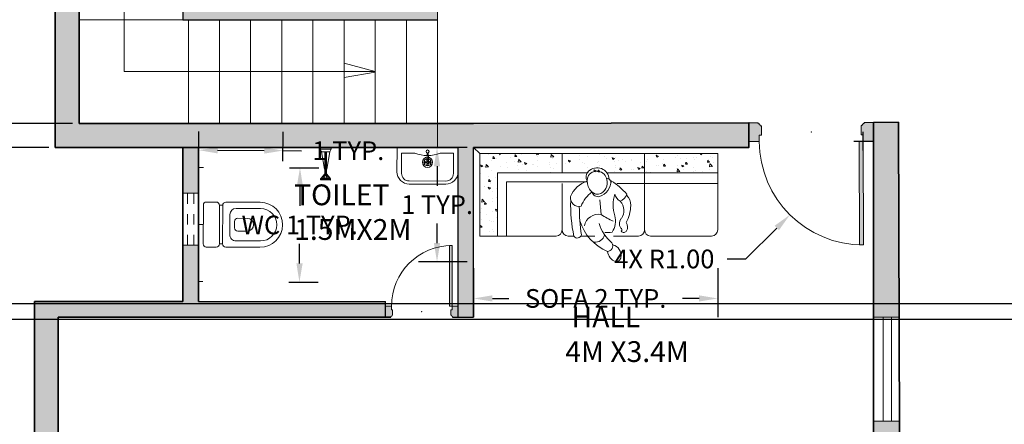
# Model space of a CAD drawing. Units: metres. Extents: x 2031 to 2061.8, y 1886.4 to 1909.8.
# Tile 3 of 10: x 2036.4 to 2045.9, y 1892.7 to 1896.6. Entities that reach past the tile are written whole.
import ezdxf

# ---------------------------------------------------------------- set-up
doc = ezdxf.new("R2010")
doc.units = ezdxf.units.M
doc.linetypes.add('DASHED', pattern=[0.75, 0.5, -0.25])
for name, color, linetype, lineweight in [('A-ANNO-DIMS', 2, 'Continuous', 18), ('A-AREA-IDEN', 7, 'Continuous', 18), ('A-FLOR-FIXT', 8, 'Continuous', 18), ('A-FLOR-STRS', 7, 'Continuous', 18), ('A-FLOR-STRS-PATH', 1, 'Continuous', 13), ('A-GLAZ-OVHD', 30, 'DASHED', 13), ('A-WALL-PATT', 252, 'Continuous', 13), ('doors & windows', 30, 'Continuous', 18), ('furniture', 24, 'Continuous', 13), ('inner walls', 4, 'Continuous', 25), ('windows', 30, 'Continuous', 18)]:
    doc.layers.add(name, color=color, linetype=linetype, lineweight=lineweight)
doc.layers.add('outer walls', color=1, linetype='Continuous', lineweight=35, plot=False)
doc.styles.get("Standard").update_dxf_attribs({"font": 'arial.ttf'})
doc.dimstyles.get("Standard").update_dxf_attribs({"dimtxt": 0.18, "dimasz": 0.18, "dimexe": 0.18, "dimexo": 0.0625, "dimgap": 0.09, "dimtad": 0, "dimtih": 1, "dimtoh": 1, "dimdec": 4, "dimzin": 0, "dimdsep": 46, "dimtxsty": 'Standard', "dimcen": 0.09, "dimadec": 0, "dimazin": 0, "dimtfac": 1, "dimtdec": 4, "dimtofl": 0, "dimtmove": 0, "dimatfit": 3, "dimfxl": 1, "dimtolj": 1, "dimtzin": 0, "dimarcsym": 0})

# ---------------------------------------------------------------- blocks, each defined once
blk = doc.blocks.new('D2')
at = {"layer": 'doors & windows'}
h = blk.add_hatch(dxfattribs=at)
h.set_pattern_fill('DOTS', color=256, scale=2, angle=180, style=0)
h.set_pattern_definition([(180, (0, -4), (-0.0625, -0.125), [0, -0.125])])
h.paths.add_polyline_path([(2.5, 0), (3.5, 0), (3.5, 24.98, 0.010003), (2.5, 25)])
h = blk.add_hatch(dxfattribs=at)
h.set_pattern_fill('DOTS', color=256, scale=2, angle=180, style=0)
h.set_pattern_definition([(180, (0, 0), (-0.0625, -0.125), [0, -0.125])])
edge = h.paths.add_edge_path()
edge.add_line((27.5, 0), (27.5, -1.5))
edge.add_line((27.5, -1.5), (27, -1.5))
edge.add_line((27, -1.5), (27, -3.75))
edge.add_line((27, -3.75), (27.25, -3.75))
edge.add_arc((27.76, -3.74), 0.509, 181.0059, 268.9941)
edge.add_line((27.75, -4.25), (27.75, -4.5))
edge.add_line((27.75, -4.5), (30, -4.5))
edge.add_line((30, -4.5), (30, 0))
edge.add_line((30, 0), (27.5, 0))
edge = h.paths.add_edge_path()
edge.add_line((2.5, -1.5), (2.5, 0))
edge.add_line((2.5, 0), (0, 0))
edge.add_line((0, 0), (0, -4.5))
edge.add_line((0, -4.5), (2.25, -4.5))
edge.add_line((2.25, -4.5), (2.25, -4.25))
edge.add_arc((2.24, -3.74), 0.509, 271.0059, 358.9941)
edge.add_line((2.75, -3.75), (3, -3.75))
edge.add_line((3, -3.75), (3, -1.5))
edge.add_line((3, -1.5), (2.5, -1.5))
for p, q in [((0, 0), (0, -4.5)), ((30, 0), (30, -4.5))]:
    blk.add_line(p, q)
blk.add_lwpolyline([(3.5, 0), (3.5, 25), (2.5, 25), (2.5, 0)], close=True, dxfattribs=at)
for points in [[(3, -3.75), (3, -1.5), (2.5, -1.5), (2.5, 0), (0, 0)], [(27, -3.75), (27, -1.5), (27.5, -1.5), (27.5, 0), (30, 0)], [(0, -4.5), (2.25, -4.5)], [(30, -4.5), (27.75, -4.5)]]:
    blk.add_lwpolyline(points, dxfattribs=at)
for points in [[(2.25, -4.5), (2.25, -4.25, 0.403966), (2.75, -3.75), (3, -3.75)], [(27.75, -4.5), (27.75, -4.25, -0.403966), (27.25, -3.75), (27, -3.75)]]:
    blk.add_lwpolyline(points, format="xyb", dxfattribs=at)
at = {"layer": 'doors & windows', "ltscale": 6}
blk.add_arc((2.5, 0), 25, 0, 90, dxfattribs=at)
at = {"layer": 'doors & windows'}
blk.add_point((15, -2.25), dxfattribs=at)
blk = doc.blocks.new('MAN')
at = {"layer": 'doors & windows'}
blk.add_line((1.3, -9.85), (0.89, -5.45), dxfattribs=at)
for centre, radius, start, end in [((-0.81, 1.3), 2.37, 132.7993, 210.1219), ((0, 0), 3.06, 359.7942, 144.0351), ((0.1, 0.48), 3.6, 2.8928, 134.5528), ((-0.36, -7.56), 8.07, 108.0153, 157.5724), ((1.3, 0.05), 4.16, 155.2349, 248.5051), ((-0.98, 0.55), 5.34, 289.2819, 356.6237), ((2.86, -0.44), 1.38, 352.7443, 87.7525), ((-8.99, -19.77), 24.04, 41.647, 56.3067), ((-0.1, -0.61), 3.22, 267.7788, 10.6507), ((-5.32, -4.92), 2.54, 170.002, 284.7527), ((34.75, -7.19), 42.53, 177.9613, 192.4551), ((4.14, -10.82), 9.46, 125.6851, 158.6987), ((0.38, -2.75), 1.79, 192.3382, 283.0231), ((15.87, -7.04), 10.97, 162.7002, 196.7262), ((8.59, -3.01), 3.29, 193.5598, 239.9446), ((5.83, -2.73), 3.32, 289.6374, 341.2911), ((3.84, -8.67), 4.24, 325.4363, 41.8446), ((6.12, -7.03), 4.01, 358.2671, 46.939), ((54.76, -7.35), 59.95, 180.1044, 188.2297), ((-0.78, -6.94), 10.91, 330.7562, 358.8997), ((9.03, -7.36), 14.72, 197.1765, 246.7641), ((0.5, -14.05), 4.27, 79.2575, 168.509), ((16.49, 13.41), 27.78, 236.8487, 245.427), ((-0.19, -11.81), 5.78, 325.2412, 16.1794), ((8.85, -12.54), 2.12, 136.0875, 215.1077), ((12.84, -8.62), 12.77, 197.9012, 229.3504), ((6.8, -14.37), 0.689, 315.9836, 61.7947), ((7.06, -13.61), 2.15, 328.4119, 38.6474), ((-5.78, -15.61), 1.25, 217.214, 345.0614), ((-0.4, -15.27), 2.81, 261.6005, 345.5998), ((3.21, -8.72), 6.53, 262.8142, 281.931), ((8.05, -14.12), 1.05, 224.0636, 323.687), ((3.09, -19.2), 1.68, 274.444, 31.8659), ((4.09, -22.01), 3.16, 349.15, 77.9716), ((6.99, -20.36), 3.8, 187.9766, 248.0432), ((5.75, -22.44), 1.45, 262.6631, 353.5986)]:
    blk.add_arc(centre, radius, start, end, dxfattribs=at)
blk = doc.blocks.new('sofa 2')
at = {"layer": 'furniture', "ltscale": 0.5}
h = blk.add_hatch(dxfattribs=at)
h.set_pattern_fill('AR-CONC', color=256, angle=450, style=0)
h.set_pattern_definition([(40, (-1099.1507, 871.655), (-0.627521, 7.172602), [0.75, -8.25]), (95, (-1099.151, 871.655), (7.52192, -1.387513), [0.6, -6.6]), (349.5486, (-1099.203, 872.253), (6.894395, 5.785094), [0.637402, -7.01142]), (43.8158, (-1097.151, 871.655), (-1.65519, 10.67241), [1.125, -12.375]), (353.3644, (-1097.289, 872.544), (9.74118, 9.34663), [0.9561, -10.51713]), (98.8158, (-1097.151, 871.655), (9.74119, 9.34662), [0.9, -9.9]), (69, (-1097.6507, 872.655), (-4.02619, 5.96907), [0.75, -8.25]), (124, (-1097.651, 872.655), (7.2515, 2.433153), [0.6, -6.6]), (18.5486, (-1097.986, 873.1524), (3.225305, 8.402226), [0.637402, -7.01142]), (52.5, (-1099.1507, 871.655), (3.3289385, 0.1215986), [0, -6.52, 0, -6.7, 0, -6.625]), (82.5, (-1099.1507, 871.655), (3.944117, 2.630695), [0, -3.82, 0, -6.37, 0, -2.525]), (122.5, (-1099.1507, 869.425), (-0.2255487, 5.3382244), [0, -2.5, 0, -7.8, 0, -10.35]), (132.5, (-1099.1507, 868.425), (1.00105, 5.831862), [0, -3.25, 0, -5.18, 0, -7.35])])
h.paths.add_polyline_path([(-8.27, -37.7, 0.168872), (-7.9, -36.76, 0.613808), (-6.95, -30.77, 0.074869), (-8.27, -30.38), (-8.27, -29), (-2, -29), (-2, -56), (-8.27, -56)])
h.paths.add_polyline_path([(-8.27, -7.77), (-29, -7.77), (-29, -2), (-2, -2), (-2, -29), (-8.27, -29)])
h.paths.add_polyline_path([(-8.27, -80), (-2, -80), (-2, -56), (-8.27, -56)])
at = {"layer": 'furniture'}
for p, q in [((-2, -2), (0, 0)), ((-29, -2), (-2, -2)), ((-29, -27), (-29, -2)), ((-2, -2), (-2, -80)), ((-8.27, -7.77), (-29, -7.77)), ((-8.27, -37.27), (-8.27, -7.77)), ((-11.27, -10.77), (-29, -10.77)), ((-11.27, -37.27), (-11.27, -10.77)), ((-27, -29), (-11.8, -29)), ((-8.27, -29), (-2, -29)), ((-29, -32.87), (-29, -31)), ((-29, -39.74), (-29, -35.16)), ((-8.27, -37.7), (-8.27, -37.7)), ((-8.27, -43.66), (-8.27, -80)), ((-29, -45.8), (-29, -54)), ((-11.8, -80), (-11.8, -46.89)), ((-29, -78), (-29, -58)), ((-27, -56), (-2, -56)), ((-2, -80), (-27, -80))]:
    blk.add_line(p, q, dxfattribs=at)
for centre, start, end in [((-27, -27), 180, 270), ((-27, -31), 90, 180), ((-27, -54), 180, 270), ((-27, -58), 90, 180), ((-27, -78), 180, 270)]:
    blk.add_arc(centre, 2, start, end, dxfattribs=at)
at = {"xscale": 1.099999999999999, "yscale": 1.099999999999999, "zscale": 1.099999999999999, "rotation": 270}
blk.add_blockref('MAN', (-11.13, -40.34), dxfattribs=at)
blk = doc.blocks.new('commode')
for p, q in [((-7.09, 19.41), (-7.09, 8.61)), ((-5.09, 11.81), (-5.09, 19.57)), ((5.09, 11.81), (5.09, 19.57)), ((7.09, 19.41), (7.09, 8.61)), ((-2, 12.37), (-2, 15.37)), ((2, 12.37), (2, 15.37)), ((-3.15, 9.87), (3.15, 9.87)), ((-1, 11.37), (1, 11.37)), ((-6.09, 7.61), (6.09, 7.61)), ((-6.09, 6.61), (-6.09, 7.61)), ((-6.09, 6.61), (6.09, 6.61)), ((6.09, 7.61), (6.09, 6.61)), ((-7.09, 2.5), (-7.09, 5.61)), ((7.09, 2.5), (7.09, 5.61)), ((-18, 1.5), (-18, 0)), ((-6.09, 1.5), (6.09, 1.5)), ((0, 1.5), (0, 0)), ((18, 1.5), (18, 0))]:
    blk.add_line(p, q)
for centre, radius, start, end in [((0, 19.41), 7.09, 0, 180), ((0, 19.57), 5.09, 0, 180), ((0, 15.37), 2, 0, 180), ((-3.15, 11.81), 1.94, 180, 270), ((-1, 12.37), 1, 180, 270), ((1, 12.37), 1, 270, 0), ((3.15, 11.81), 1.94, 270, 0), ((-6.09, 8.61), 1, 180, 270), ((-6.09, 5.61), 1, 90, 180), ((6.09, 8.61), 1, 270, 0), ((6.09, 5.61), 1, 0, 90), ((-6.09, 2.5), 1, 180, 270), ((6.09, 2.5), 1, 270, 0)]:
    blk.add_arc(centre, radius, start, end)
blk = doc.blocks.new('wash basin 1')
for p, q in [((0, 10), (-8, 10)), ((0, 10), (0, -10)), ((-8.5, 8.5), (-1.85, 8.5)), ((-1.85, 8.5), (-1.85, 4.19)), ((-12, 6), (-12, -6)), ((-11, 6), (-11, -6)), ((-1.85, -8.5), (-1.85, -4.19)), ((-8.5, -8.5), (-1.85, -8.5)), ((0, -10), (-8, -10))]:
    blk.add_line(p, q)
blk.add_lwpolyline([(-1.83, 0.11), (-5.25, 0.25), (-5.23, -0.38), (-1.8, -0.19)])
for centre, radius in [((-4.87, 0), 1.68), ((-4.87, 0), 1.18), ((-5.63, 0), 0.25), ((-4.87, 0.75), 0.25), ((-4.87, 0), 0.25), ((-4.19, 0), 0.25), ((-1.34, 0), 0.5), ((-4.87, -0.72), 0.25)]:
    blk.add_circle(centre, radius)
for centre, radius, start, end in [((-8, 6), 4, 90, 180), ((-8.5, 6), 2.5, 90, 180), ((8.89, 0), 11.53, 158.7059, 201.2941), ((-8, -6), 4, 180, 270), ((-8.5, -6), 2.5, 180, 270)]:
    blk.add_arc(centre, radius, start, end)
blk = doc.blocks.new('tap & shower')
for p, q in [((1.71, 0), (-1.71, 0)), ((-1.71, 0), (-1.71, -0.5)), ((1.71, 0), (1.71, -0.5)), ((1.71, -0.5), (-1.71, -0.5)), ((1.31, -1.4), (-1.31, -1.4)), ((-1.31, -1.4), (-0.39, -7)), ((-0.32, -0.5), (0.32, -0.5)), ((-0.27, -7.94), (-0.27, -1.4)), ((-0.22, -7.94), (-0.22, -1.4)), ((-0.16, -7.94), (-0.16, -1.4)), ((0, -8.48), (0, -1.4)), ((0.16, -7.94), (0.16, -1.4)), ((0.22, -7.94), (0.22, -1.4)), ((0.27, -7.94), (0.27, -1.4)), ((0.39, -7), (1.31, -1.4)), ((-1.48, -9.96), (-0.27, -8.48)), ((-0.21, -8.48), (-0.94, -9.96)), ((-0.09, -8.48), (-0.4, -9.96)), ((-0.32, -7.94), (0.32, -7.94)), ((-0.32, -8.48), (-0.32, -7.94)), ((-0.32, -8.48), (0.32, -8.48)), ((0.09, -8.48), (0.4, -9.96)), ((0.21, -8.48), (0.94, -9.96)), ((1.48, -9.96), (0.27, -8.48)), ((0.32, -8.48), (0.32, -7.94)), ((-1.62, -10.37), (-1.62, -10.1)), ((-1.48, -9.96), (1.48, -9.96)), ((-1.48, -10.5), (-1.48, -9.96)), ((-1.48, -10.5), (1.48, -10.5)), ((-1.43, -10.5), (-1.43, -9.96)), ((-1.37, -10.5), (-1.37, -9.96)), ((-1.32, -10.5), (-1.32, -9.96)), ((-1.27, -10.5), (-1.27, -9.96)), ((-1.21, -10.5), (-1.21, -9.96)), ((-1.16, -10.5), (-1.16, -9.96)), ((-1.1, -10.5), (-1.1, -9.96)), ((-1.05, -10.5), (-1.05, -9.96)), ((-1, -10.5), (-1, -9.96)), ((-0.94, -10.5), (-0.94, -9.96)), ((-0.89, -10.5), (-0.89, -9.96)), ((-0.84, -10.5), (-0.84, -9.96)), ((-0.78, -10.5), (-0.78, -9.96)), ((-0.73, -10.5), (-0.73, -9.96)), ((-0.67, -10.5), (-0.67, -9.96)), ((-0.62, -10.5), (-0.62, -9.96)), ((-0.57, -10.5), (-0.57, -9.96)), ((-0.51, -10.5), (-0.51, -9.96)), ((-0.46, -10.5), (-0.46, -9.96)), ((-0.4, -10.5), (-0.4, -9.96)), ((-0.35, -10.5), (-0.35, -9.96)), ((-0.3, -10.5), (-0.3, -9.96)), ((-0.24, -10.5), (-0.24, -9.96)), ((-0.19, -10.5), (-0.19, -9.96)), ((-0.13, -10.5), (-0.13, -9.96)), ((-0.08, -10.5), (-0.08, -9.96)), ((-0.03, -10.5), (-0.03, -9.96)), ((0.03, -10.5), (0.03, -9.96)), ((0.08, -10.5), (0.08, -9.96)), ((0.13, -10.5), (0.13, -9.96)), ((0.19, -10.5), (0.19, -9.96)), ((0.24, -10.5), (0.24, -9.96)), ((0.3, -10.5), (0.3, -9.96)), ((0.35, -10.5), (0.35, -9.96)), ((0.4, -10.5), (0.4, -9.96)), ((0.46, -10.5), (0.46, -9.96)), ((0.51, -10.5), (0.51, -9.96)), ((0.57, -10.5), (0.57, -9.96)), ((0.62, -10.5), (0.62, -9.96)), ((0.67, -10.5), (0.67, -9.96)), ((0.73, -10.5), (0.73, -9.96)), ((0.78, -10.5), (0.78, -9.96)), ((0.84, -10.5), (0.84, -9.96)), ((0.89, -10.5), (0.89, -9.96)), ((0.94, -10.5), (0.94, -9.96)), ((1, -10.5), (1, -9.96)), ((1.05, -10.5), (1.05, -9.96)), ((1.1, -10.5), (1.1, -9.96)), ((1.16, -10.5), (1.16, -9.96)), ((1.21, -10.5), (1.21, -9.96)), ((1.27, -10.5), (1.27, -9.96)), ((1.32, -10.5), (1.32, -9.96)), ((1.37, -10.5), (1.37, -9.96)), ((1.43, -10.5), (1.43, -9.96)), ((1.48, -10.5), (1.48, -9.96)), ((1.62, -10.37), (1.62, -10.1))]:
    blk.add_line(p, q)
for centre, radius, start, end in [((-0.02, -0.29), 1.7, 187.1825, 220.9028), ((0.02, -0.29), 1.7, 319.0972, 352.8175), ((0, -6.99), 0.392, 181.7992, 358.2008), ((-1.48, -10.1), 0.135, 90, 180), ((-1.48, -10.37), 0.135, 180, 270), ((1.48, -10.1), 0.135, 0, 90), ((1.48, -10.37), 0.135, 270, 0)]:
    blk.add_arc(centre, radius, start, end)
blk = doc.blocks.new('*D30')
at = {"layer": 'A-ANNO-DIMS', "color": 0, "lineweight": -2, "transparency": 16777216}
for p, q in [((2038.9882, 1895.1459), (2039.2707, 1895.1445)), ((2039.0898, 1894.9654), (2039.0889, 1894.7784)), ((2039.0862, 1894.2253), (2039.0871, 1894.4123)), ((2038.9828, 1894.0458), (2039.2653, 1894.0444))]:
    blk.add_line(p, q, dxfattribs=at)
at = {"layer": 'A-ANNO-DIMS', "color": 0, "transparency": 16777216}
for points in [[(2039.0598, 1894.9655), (2039.1198, 1894.9652), (2039.0907, 1895.1454)], [(2039.0562, 1894.2254), (2039.1162, 1894.2251), (2039.0853, 1894.0453)]]:
    blk.add_solid(points, dxfattribs=at)
at = {"layer": 'Defpoints', "color": 0, "transparency": 16777216}
for p in [(2038.9257, 1895.1462), (2038.9203, 1894.0461), (2039.0853, 1894.0453)]:
    blk.add_point(p, dxfattribs=at)
at = {"layer": 'A-ANNO-DIMS', "color": 0, "transparency": 16777216, "insert": (2039.088, 1894.5953), "char_height": 0.18, "attachment_point": 5}
blk.add_mtext('\\A1;WC 1 TYP.', dxfattribs=at)
blk = doc.blocks.new('*D31')
at = {"layer": 'A-ANNO-DIMS', "color": 0, "lineweight": -2, "transparency": 16777216}
for p, q in [((2038.1162, 1895.2127), (2038.1176, 1895.4952)), ((2038.926, 1895.2087), (2038.9274, 1895.4912)), ((2038.2967, 1895.3143), (2038.7465, 1895.3121)), ((2038.9265, 1895.3112), (2039.1065, 1895.3103))]:
    blk.add_line(p, q, dxfattribs=at)
at = {"layer": 'A-ANNO-DIMS', "color": 0, "transparency": 16777216}
for points in [[(2038.2969, 1895.3443), (2038.2966, 1895.2843), (2038.1167, 1895.3152)], [(2038.7467, 1895.3421), (2038.7464, 1895.2821), (2038.9265, 1895.3112)]]:
    blk.add_solid(points, dxfattribs=at)
at = {"layer": 'Defpoints', "color": 0, "transparency": 16777216}
for p in [(2038.9265, 1895.3112), (2038.1159, 1895.1502), (2038.9257, 1895.1462)]:
    blk.add_point(p, dxfattribs=at)
at = {"layer": 'A-ANNO-DIMS', "color": 0, "transparency": 16777216, "insert": (2039.5562, 1895.3103), "char_height": 0.18, "attachment_point": 5}
blk.add_mtext('\\A1;1 TYP.', dxfattribs=at)
blk = doc.blocks.new('*D34')
at = {"layer": 'A-ANNO-DIMS', "color": 0, "lineweight": -2, "transparency": 16777216}
for p, q in [((2040.7632, 1894.1783), (2040.7632, 1893.7082)), ((2043.1138, 1894.1783), (2043.1138, 1893.7082)), ((2040.9432, 1893.8882), (2041.1035, 1893.8882)), ((2042.9338, 1893.8882), (2042.7735, 1893.8882))]:
    blk.add_line(p, q, dxfattribs=at)
at = {"layer": 'A-ANNO-DIMS', "color": 0, "transparency": 16777216}
for points in [[(2040.9432, 1893.9182), (2040.9432, 1893.8582), (2040.7632, 1893.8882)], [(2042.9338, 1893.9182), (2042.9338, 1893.8582), (2043.1138, 1893.8882)]]:
    blk.add_solid(points, dxfattribs=at)
at = {"layer": 'Defpoints', "color": 0, "transparency": 16777216}
for p in [(2040.7632, 1894.2408), (2043.1138, 1894.2408), (2040.7632, 1893.8882)]:
    blk.add_point(p, dxfattribs=at)
at = {"layer": 'A-ANNO-DIMS', "color": 0, "transparency": 16777216, "insert": (2041.9385, 1893.8882), "char_height": 0.18, "attachment_point": 5}
blk.add_mtext('\\A1;SOFA 2 TYP.', dxfattribs=at)
blk = doc.blocks.new('*D35')
at = {"layer": 'A-ANNO-DIMS', "color": 0, "lineweight": -2, "transparency": 16777216}
for p, q in [((2040.7007, 1895.3412), (2040.2306, 1895.3412)), ((2040.4106, 1895.1612), (2040.4106, 1894.9714)), ((2040.4106, 1894.4208), (2040.4106, 1894.6106)), ((2040.7007, 1894.2408), (2040.2306, 1894.2408))]:
    blk.add_line(p, q, dxfattribs=at)
at = {"layer": 'A-ANNO-DIMS', "color": 0, "transparency": 16777216}
for points in [[(2040.3806, 1895.1612), (2040.4406, 1895.1612), (2040.4106, 1895.3412)], [(2040.3806, 1894.4208), (2040.4406, 1894.4208), (2040.4106, 1894.2408)]]:
    blk.add_solid(points, dxfattribs=at)
at = {"layer": 'Defpoints', "color": 0, "transparency": 16777216}
for p in [(2040.4106, 1895.3412), (2040.7632, 1895.3412), (2040.7632, 1894.2408)]:
    blk.add_point(p, dxfattribs=at)
at = {"layer": 'A-ANNO-DIMS', "color": 0, "transparency": 16777216, "insert": (2040.4106, 1894.791), "char_height": 0.18, "attachment_point": 5}
blk.add_mtext('\\A1;1 TYP.', dxfattribs=at)
blk = doc.blocks.new('*D44')
at = {"layer": 'A-ANNO-DIMS', "color": 0, "lineweight": -2, "transparency": 16777216}
for p, q in [((2036.2328, 1900.7199), (2036.2328, 1886.3902)), ((2056.4539, 1889.9931), (2056.4539, 1886.3902)), ((2036.4128, 1886.5702), (2045.949, 1886.5702)), ((2056.2739, 1886.5702), (2046.7377, 1886.5702))]:
    blk.add_line(p, q, dxfattribs=at)
at = {"layer": 'A-ANNO-DIMS', "color": 0, "transparency": 16777216}
for points in [[(2036.4128, 1886.6002), (2036.4128, 1886.5402), (2036.2328, 1886.5702)], [(2056.2739, 1886.6002), (2056.2739, 1886.5402), (2056.4539, 1886.5702)]]:
    blk.add_solid(points, dxfattribs=at)
at = {"layer": 'Defpoints', "color": 0, "transparency": 16777216}
for p in [(2036.2328, 1900.7824), (2056.4539, 1890.0556), (2056.4539, 1886.5702)]:
    blk.add_point(p, dxfattribs=at)
at = {"layer": 'A-ANNO-DIMS', "color": 0, "transparency": 16777216, "insert": (2046.3433, 1886.5702), "char_height": 0.18, "attachment_point": 5}
blk.add_mtext('\\A1;20.22', dxfattribs=at)
blk = doc.blocks.new('*D51')
at = {"layer": 'A-ANNO-DIMS', "color": 0, "lineweight": -2, "transparency": 16777216}
for p, q in [((2036.9007, 1899.3712), (2031.5648, 1899.3712)), ((2031.7448, 1899.1912), (2031.7448, 1897.6532)), ((2031.7448, 1895.7512), (2031.7448, 1897.2892)), ((2036.9007, 1895.5712), (2031.5648, 1895.5712))]:
    blk.add_line(p, q, dxfattribs=at)
at = {"layer": 'A-ANNO-DIMS', "color": 0, "transparency": 16777216}
for points in [[(2031.7148, 1899.1912), (2031.7748, 1899.1912), (2031.7448, 1899.3712)], [(2031.7148, 1895.7512), (2031.7748, 1895.7512), (2031.7448, 1895.5712)]]:
    blk.add_solid(points, dxfattribs=at)
at = {"layer": 'Defpoints', "color": 0, "transparency": 16777216}
for p in [(2031.7448, 1899.3712), (2036.9632, 1899.3712), (2036.9632, 1895.5712)]:
    blk.add_point(p, dxfattribs=at)
at = {"layer": 'A-ANNO-DIMS', "color": 0, "transparency": 16777216, "insert": (2031.7448, 1897.4712), "char_height": 0.18, "attachment_point": 5}
blk.add_mtext('\\A1;3.8', dxfattribs=at)
blk = doc.blocks.new('*D54')
at = {"layer": 'A-ANNO-DIMS', "color": 0, "lineweight": -2, "transparency": 16777216}
for p, q in [((2036.6707, 1895.3412), (2031.5648, 1895.3412)), ((2031.7448, 1895.1612), (2031.7448, 1892.892)), ((2031.7448, 1890.2591), (2031.7448, 1892.5282)), ((2036.4707, 1890.0791), (2031.5648, 1890.0791))]:
    blk.add_line(p, q, dxfattribs=at)
at = {"layer": 'A-ANNO-DIMS', "color": 0, "transparency": 16777216}
for points in [[(2031.7148, 1895.1612), (2031.7748, 1895.1612), (2031.7448, 1895.3412)], [(2031.7148, 1890.2591), (2031.7748, 1890.2591), (2031.7448, 1890.0791)]]:
    blk.add_solid(points, dxfattribs=at)
at = {"layer": 'Defpoints', "color": 0, "transparency": 16777216}
for p in [(2036.7332, 1895.3412), (2031.7448, 1890.0791), (2036.5332, 1890.0791)]:
    blk.add_point(p, dxfattribs=at)
at = {"layer": 'A-ANNO-DIMS', "color": 0, "transparency": 16777216, "insert": (2031.7448, 1892.7101), "char_height": 0.18, "attachment_point": 5}
blk.add_mtext('\\A1;5.262', dxfattribs=at)
blk = doc.blocks.new('*D61')
at = {"layer": 'A-ANNO-DIMS', "color": 0, "lineweight": -2, "transparency": 16777216}
for p, q in [((2031.7448, 1894.0148), (2031.7448, 1894.1948)), ((2031.7448, 1894.1948), (2031.9248, 1894.1948)), ((2052.1275, 1893.8348), (2031.5648, 1893.8348)), ((2051.9775, 1893.6848), (2031.5648, 1893.6848)), ((2031.7448, 1893.5048), (2031.7448, 1893.3248))]:
    blk.add_line(p, q, dxfattribs=at)
at = {"layer": 'A-ANNO-DIMS', "color": 0, "transparency": 16777216}
for points in [[(2031.7148, 1894.0148), (2031.7748, 1894.0148), (2031.7448, 1893.8348)], [(2031.7148, 1893.5048), (2031.7748, 1893.5048), (2031.7448, 1893.6848)]]:
    blk.add_solid(points, dxfattribs=at)
at = {"layer": 'Defpoints', "color": 0, "transparency": 16777216}
for p in [(2031.7448, 1893.8348), (2052.19, 1893.8348), (2052.04, 1893.6848)]:
    blk.add_point(p, dxfattribs=at)
at = {"layer": 'A-ANNO-DIMS', "color": 0, "transparency": 16777216, "insert": (2032.2492, 1894.1948), "char_height": 0.18, "attachment_point": 5}
blk.add_mtext('\\A1;0.15', dxfattribs=at)
blk = doc.blocks.new('*D64')
at = {"layer": 'A-ANNO-DIMS', "color": 0, "lineweight": -2, "transparency": 16777216}
for p, q in [((2044.5141, 1895.3129), (2044.5141, 1895.4929)), ((2044.4241, 1895.4029), (2044.6041, 1895.4029)), ((2043.3857, 1894.2683), (2043.6819, 1894.5662)), ((2043.2057, 1894.2683), (2043.3857, 1894.2683))]:
    blk.add_line(p, q, dxfattribs=at)
at = {"layer": 'A-ANNO-DIMS', "color": 0, "transparency": 16777216}
blk.add_solid([(2043.6606, 1894.5873), (2043.7032, 1894.545), (2043.8088, 1894.6938)], dxfattribs=at)
at = {"layer": 'Defpoints', "color": 0, "transparency": 16777216}
for p in [(2044.5141, 1895.4029), (2043.8088, 1894.6938)]:
    blk.add_point(p, dxfattribs=at)
at = {"layer": 'A-ANNO-DIMS', "color": 0, "transparency": 16777216, "insert": (2042.5991, 1894.2683), "char_height": 0.18, "attachment_point": 5}
blk.add_mtext('\\A1;4X R1.00', dxfattribs=at)

msp = doc.modelspace()

# ---------------------------------------------------------------- hatches: boundary and pattern name
at = {"layer": 'A-WALL-PATT'}
h = msp.add_hatch(color=256, dxfattribs=at)
h.dxf.hatch_style = 1
h.paths.add_polyline_path([(2036.9632, 1899.3712), (2037.9632, 1899.3712), (2037.9631, 1899.6012), (2036.7332, 1899.6012), (2036.7332, 1895.3412), (2040.4157, 1895.3412), (2040.4157, 1895.5712), (2038.0157, 1895.5712), (2036.9632, 1895.5712), (2036.9632, 1896.5712), (2036.9632, 1898.3712)])
h.paths.add_polyline_path([(2038.0632, 1898.2712), (2040.4157, 1898.2712), (2040.4157, 1898.3712), (2037.9632, 1898.3712), (2037.9632, 1896.5712), (2040.4157, 1896.5712), (2040.4157, 1896.6712), (2038.0632, 1896.6712)], flags=17)
h = msp.add_hatch(color=256, dxfattribs=at)
h.dxf.hatch_style = 1
h.paths.add_polyline_path([(2036.7632, 1893.709), (2039.9132, 1893.709), (2039.9132, 1893.859), (2038.1132, 1893.859), (2038.1132, 1894.4001), (2037.9632, 1894.4001), (2037.9632, 1893.859), (2036.5332, 1893.859), (2036.5332, 1892.3865), (2036.7632, 1892.3865)])
h.paths.add_polyline_path([(2038.1132, 1895.3412), (2037.9632, 1895.3412), (2037.9632, 1894.9001), (2038.1132, 1894.9001)])
h.paths.add_polyline_path([(2043.4132, 1895.5795), (2040.7632, 1895.5712), (2040.4157, 1895.5712), (2040.4157, 1895.3412), (2040.6132, 1895.3412), (2040.6132, 1893.709), (2040.7632, 1893.709), (2040.7632, 1895.3412), (2043.4139, 1895.3412)])
h.paths.add_polyline_path([(2039.7057, 1890.309), (2036.7632, 1890.309), (2036.7632, 1891.1865), (2036.5332, 1891.1865), (2036.5332, 1890.079), (2038.4982, 1890.079), (2038.4982, 1888.429), (2038.6482, 1888.429), (2038.6482, 1890.079), (2039.7057, 1890.079)])
h.paths.add_polyline_path([(2042.7749, 1889.8182), (2042.6136, 1889.8182), (2042.6136, 1891.8182), (2042.6136, 1891.9682), (2042.4636, 1891.9682), (2041.6986, 1891.9682), (2041.6986, 1891.8182), (2042.4636, 1891.8182), (2042.4636, 1889.8182), (2041.2982, 1889.8182), (2041.2982, 1890.309), (2041.1482, 1890.309), (2041.1482, 1888.429), (2041.2982, 1888.429), (2041.2982, 1889.5882), (2042.7749, 1889.5882)])
h.paths.add_polyline_path([(2044.8641, 1892.708), (2044.6136, 1892.708), (2044.6136, 1891.9682), (2044.0858, 1891.9682), (2044.0858, 1891.8182), (2044.5977, 1891.8182), (2044.6136, 1891.8182), (2044.6136, 1889.8182), (2043.7749, 1889.8182), (2043.7749, 1889.5882), (2044.8739, 1889.5882)])
h.paths.add_polyline_path([(2044.8551, 1895.584), (2044.6136, 1895.5833), (2044.6136, 1895.5676), (2044.6141, 1895.4033), (2044.6136, 1895.4033), (2044.6136, 1893.708), (2044.8609, 1893.708)])

# ---------------------------------------------------------------- linework, layer by layer
at = {"layer": 'A-FLOR-STRS'}
for p, q in [((2040.4157, 1896.6712), (2040.4157, 1895.3412)), ((2037.9632, 1896.5712), (2036.9632, 1896.5712)), ((2038.0157, 1896.5712), (2038.0157, 1895.5712)), ((2038.3157, 1896.5712), (2038.3157, 1895.5712)), ((2038.6157, 1896.5712), (2038.6157, 1895.5712)), ((2038.9157, 1896.5712), (2038.9157, 1895.5712)), ((2039.2157, 1896.5712), (2039.2157, 1895.5712)), ((2039.5157, 1896.5712), (2039.5157, 1895.5712)), ((2039.8157, 1896.5712), (2039.8157, 1895.5712)), ((2040.1157, 1896.5712), (2040.1157, 1895.5712))]:
    msp.add_line(p, q, dxfattribs=at)
at = {"layer": 'A-FLOR-STRS-PATH'}
for p, q in [((2037.3981, 1898.8212), (2037.3981, 1896.5712)), ((2037.3981, 1896.5712), (2037.3981, 1896.0716)), ((2039.8157, 1896.0712), (2039.5157, 1896.1541)), ((2037.3981, 1896.0716), (2039.8157, 1896.0712)), ((2039.8146, 1896.0671), (2039.5157, 1896.0142))]:
    msp.add_line(p, q, dxfattribs=at)
at = {"layer": 'A-GLAZ-OVHD', "ltscale": 0.2}
for p, q in [((2038.0082, 1894.4001), (2038.0082, 1894.9001)), ((2038.0682, 1894.4001), (2038.0682, 1894.9001))]:
    msp.add_line(p, q, dxfattribs=at)
at = {"layer": 'inner walls'}
for p, q in [((2037.9632, 1898.3712), (2037.9632, 1896.5712)), ((2040.6132, 1893.709), (2040.6132, 1895.3412)), ((2040.7632, 1893.709), (2040.7632, 1895.3412)), ((2038.1132, 1893.859), (2039.9132, 1893.859)), ((2039.9132, 1893.709), (2039.9132, 1893.859)), ((2040.5607, 1893.709), (2040.7632, 1893.709))]:
    msp.add_line(p, q, dxfattribs=at)
msp.add_lwpolyline([(2037.9632, 1896.5712), (2040.4157, 1896.5712)], dxfattribs=at)
at = {"layer": 'outer walls'}
for p, q in [((2036.7332, 1899.6012), (2036.7332, 1895.3412)), ((2036.9632, 1898.3712), (2036.9632, 1896.5712)), ((2036.9632, 1896.5712), (2036.9632, 1895.5712)), ((2036.9632, 1895.5712), (2038.0157, 1895.5712)), ((2040.7632, 1895.5712), (2038.0157, 1895.5712)), ((2044.8551, 1895.584), (2044.6136, 1895.5833)), ((2044.6136, 1895.5833), (2044.6136, 1891.9682)), ((2036.7332, 1895.3412), (2040.6132, 1895.3412)), ((2037.9632, 1895.3412), (2037.9632, 1893.859)), ((2038.1132, 1895.3412), (2038.1132, 1893.859)), ((2036.5332, 1893.859), (2037.9632, 1893.859)), ((2036.5332, 1893.859), (2036.5332, 1890.079)), ((2036.7632, 1893.709), (2039.9657, 1893.709)), ((2036.7632, 1893.709), (2036.7632, 1890.309))]:
    msp.add_line(p, q, dxfattribs=at)
for points in [[(2040.7632, 1895.3412), (2043.4139, 1895.3412), (2043.4132, 1895.5795)], [(2040.7632, 1895.5712), (2043.4139, 1895.5795), (2043.4139, 1895.3412)], [(2041.2982, 1889.5882), (2044.8739, 1889.5882), (2044.8551, 1895.584)]]:
    msp.add_lwpolyline(points, dxfattribs=at)
at = {"layer": 'windows'}
for p, q in [((2038.1132, 1894.9001), (2037.9632, 1894.9001)), ((2038.1132, 1894.4001), (2037.9632, 1894.4001)), ((2044.8609, 1893.708), (2044.6136, 1893.708)), ((2044.7059, 1892.708), (2044.7059, 1893.708)), ((2044.7859, 1892.708), (2044.7859, 1893.708)), ((2044.8609, 1892.708), (2044.6136, 1892.708))]:
    msp.add_line(p, q, dxfattribs=at)

# ---------------------------------------------------------------- block references
at = {"layer": 'A-FLOR-FIXT'}
for name, p, xscale, yscale, zscale, rotation in [('tap & shower', (2039.3385, 1895.3412), -0.0297885069260649, 0.0297885069260649, 0.0297885069260649, 359.8832026368535), ('wash basin 1', (2040.3192, 1895.3418), 0.0294025239596969, 0.0294025239596969, 0.0294025239596969, 89.8832026368535), ('commode', (2038.1132, 1894.6001), 0.030558270807299, 0.030558270807299, 0.030558270807299, 269.7177447288221)]:
    msp.add_blockref(name, p, dxfattribs=dict(at, xscale=xscale, yscale=yscale, zscale=zscale, rotation=rotation))
at = {"layer": 'doors & windows', "xscale": 0.0400050437972118, "yscale": 0.0400050437972118, "zscale": 0.0400050437972118, "rotation": 180.1795979327068}
msp.add_blockref('D2', (2044.6141, 1895.4033), dxfattribs=at)
at = {"layer": 'doors & windows', "xscale": -0.0233333333333255, "yscale": 0.0233333333333255, "zscale": 0.0233333333333255}
msp.add_blockref('D2', (2040.6132, 1893.814), dxfattribs=at)
at = {"layer": 'furniture', "xscale": 0.0293822575608255, "yscale": 0.0293822575608255, "zscale": 0.0293822575608255, "rotation": 90.00000000000003}
msp.add_blockref('sofa 2', (2040.7632, 1895.3412), dxfattribs=at)

# ---------------------------------------------------------------- texts
at = {"layer": 'A-AREA-IDEN', "attachment_point": 7}
for s, width, insert, char_height in [('TOILET\\P1.5MX2M', 1.594747, (2039.0341, 1894.4518), 0.20006), ('    HALL\\P   4M X3.4M', 2.30233, (2041.462, 1893.2765), 0.2)]:
    msp.add_mtext_dynamic_manual_height_columns(s, width=width, gutter_width=12.5, heights=[0], dxfattribs=dict(at, insert=insert, char_height=char_height))

# ---------------------------------------------------------------- dimensions: what is measured, and where the dimension line sits
at = {"layer": 'A-ANNO-DIMS'}
dim = msp.add_linear_dim(base=(2056.4539, 1886.5702), p1=(2036.2328, 1900.7824), p2=(2056.4539, 1890.0556), dimstyle='Standard', override={"dimdec": 2, "dimlfac": 1, "dimrnd": 0, "dimzin": 0, "dimdsep": 46, "dimlunit": 2}, dxfattribs=at)
dim.commit()
dim.dimension.update_dxf_attribs({"geometry": '*D44', "text_midpoint": (2046.3433, 1886.5702)})
for base, p1, p2, override, picture, middle in [((2031.7448, 1899.3712), (2036.9632, 1895.5712), (2036.9632, 1899.3712), {"dimdec": 1, "dimlfac": 1, "dimrnd": 0, "dimzin": 0, "dimdsep": 46, "dimlunit": 2}, '*D51', (2031.7448, 1897.4712)), ((2031.7448, 1890.079), (2036.7332, 1895.3412), (2036.5332, 1890.079), {"dimdec": 3, "dimlfac": 1, "dimrnd": 0, "dimzin": 0, "dimdsep": 46, "dimlunit": 2}, '*D54', (2031.7448, 1892.7101)), ((2031.7448, 1893.8348), (2052.04, 1893.6848), (2052.19, 1893.8348), {"dimdec": 2, "dimlfac": 1, "dimrnd": 0, "dimzin": 0, "dimdsep": 46, "dimlunit": 2}, '*D61', (2032.2492, 1894.1948))]:
    dim = msp.add_linear_dim(base=base, p1=p1, p2=p2, angle=90, dimstyle='Standard', override=override, dxfattribs=at)
    dim.commit()
    dim.dimension.update_dxf_attribs({"geometry": picture, "text_midpoint": middle})
for base, p1, p2, angle, text, picture, middle in [((2038.9265, 1895.3112), (2038.1159, 1895.1502), (2038.9257, 1895.1462), 359.71774, '<> TYP.', '*D31', (2039.5562, 1895.3103)), ((2040.4106, 1895.3412), (2040.7632, 1894.2408), (2040.7632, 1895.3412), 90, '<> TYP.', '*D35', (2040.4106, 1894.791)), ((2039.0853, 1894.0453), (2038.9257, 1895.1462), (2038.9203, 1894.0461), 269.71774, 'WC <> TYP.', '*D30', (2039.088, 1894.5953)), ((2040.7632, 1893.8882), (2043.1138, 1894.2408), (2040.7632, 1894.2408), 180, 'SOFA <> TYP.', '*D34', (2041.9385, 1893.8882))]:
    dim = msp.add_linear_dim(base=base, p1=p1, p2=p2, angle=angle, text=text, dimstyle='Standard', override={"dimdec": 0, "dimlfac": 1, "dimrnd": 0, "dimzin": 0, "dimdsep": 46, "dimlunit": 2}, dxfattribs=at)
    dim.commit()
    dim.dimension.update_dxf_attribs({"geometry": picture, "text_midpoint": middle})
dim = msp.add_radius_dim(center=(2044.5141, 1895.4029), mpoint=(2043.8088, 1894.6938), text='4X <>', dimstyle='Standard', override={"dimdec": 2, "dimlfac": 1, "dimrnd": 0, "dimzin": 0, "dimdsep": 46, "dimlunit": 2}, dxfattribs=at)
dim.commit()
dim.dimension.update_dxf_attribs({"geometry": '*D64', "text_midpoint": (2042.5991, 1894.2683), "dimtype": 164})

doc.saveas('drawing.dxf')
